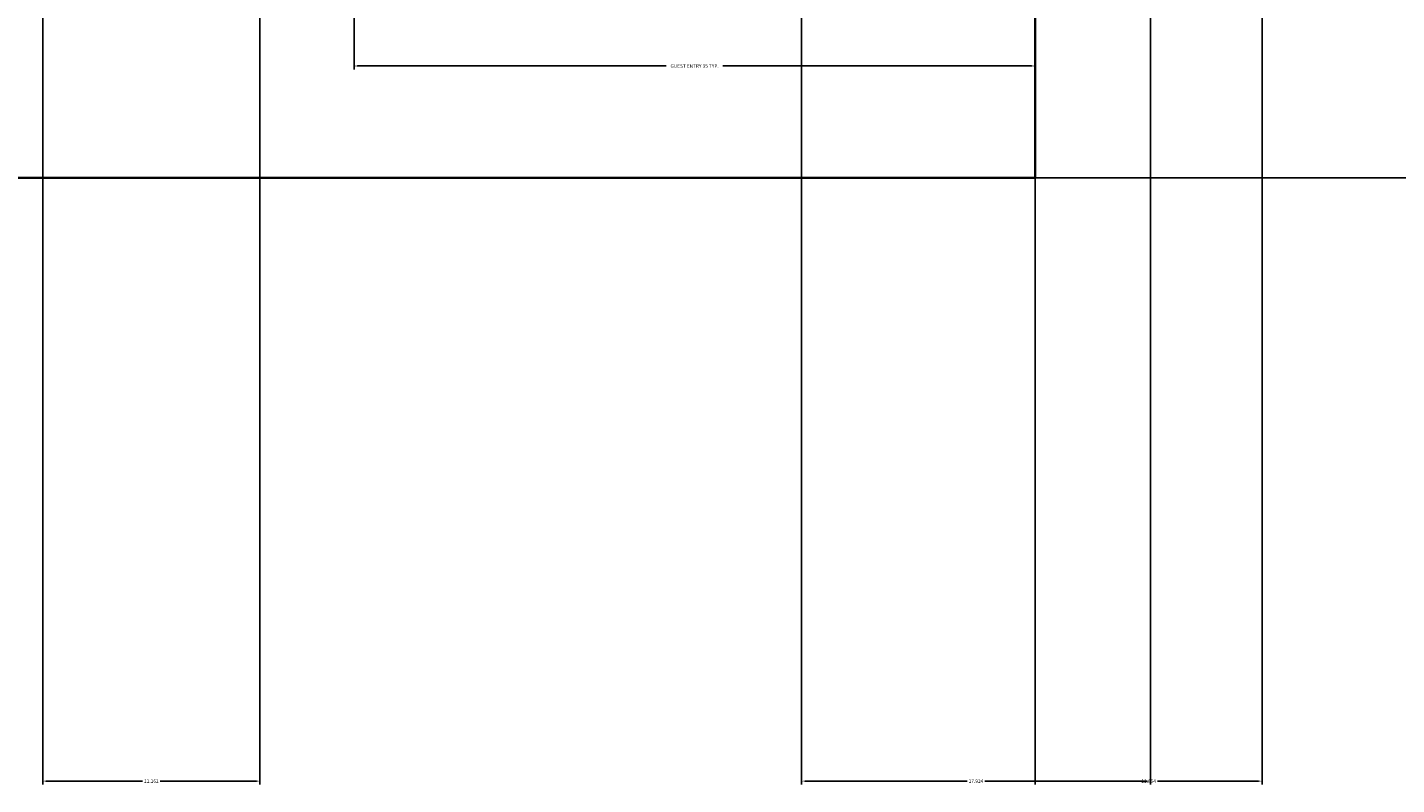
# Model space of a CAD drawing. Units: feet. Extents: x 1654 to 2985, y 1348 to 2230.
# Tile 8 of 53: x 1956 to 2027, y 1534 to 1573. Entities that reach past the tile are written whole.
import ezdxf

# ---------------------------------------------------------------- set-up
doc = ezdxf.new("R2010")
doc.units = ezdxf.units.FT
for name, color, linetype, lineweight in [('A-ANNO-DIMS', 2, 'Continuous', 18), ('A-FLOR', 7, 'Continuous', 25), ('A-WALL', 7, 'Continuous', 35)]:
    doc.layers.add(name, color=color, linetype=linetype, lineweight=lineweight)
doc.styles.get("Standard").update_dxf_attribs({"font": 'arial.ttf'})
doc.dimstyles.get("Standard").update_dxf_attribs({"dimtxt": 0.18, "dimasz": 0.18, "dimexe": 0.18, "dimexo": 0.0625, "dimgap": 0.09, "dimtad": 0, "dimtih": 1, "dimtoh": 1, "dimdec": 4, "dimzin": 0, "dimdsep": 46, "dimtxsty": 'Standard', "dimcen": 0.09, "dimadec": 0, "dimazin": 0, "dimtfac": 1, "dimtdec": 4, "dimtofl": 0, "dimtmove": 0, "dimatfit": 3, "dimfxl": 1, "dimtolj": 1, "dimtzin": 0, "dimarcsym": 0})

# ---------------------------------------------------------------- blocks, each defined once
blk = doc.blocks.new('*D30')
at = {"layer": 'A-ANNO-DIMS', "color": 0, "lineweight": -2, "transparency": 16777216}
for p, q in [((1973.092, 1576.192), (1973.092, 1570.825)), ((2008.092, 1576.192), (2008.092, 1570.825)), ((1973.272, 1571.005), (1989.137, 1571.005)), ((2007.912, 1571.005), (1992.048, 1571.005))]:
    blk.add_line(p, q, dxfattribs=at)
at = {"layer": 'A-ANNO-DIMS', "color": 0, "transparency": 16777216}
for points in [[(1973.272, 1571.035), (1973.272, 1570.975), (1973.092, 1571.005)], [(2007.912, 1571.035), (2007.912, 1570.975), (2008.092, 1571.005)]]:
    blk.add_solid(points, dxfattribs=at)
at = {"layer": 'Defpoints', "color": 0, "transparency": 16777216}
for p in [(1973.092, 1576.255), (2008.092, 1576.255), (2008.092, 1571.005)]:
    blk.add_point(p, dxfattribs=at)
at = {"layer": 'A-ANNO-DIMS', "color": 0, "transparency": 16777216, "insert": (1990.592, 1571.005), "char_height": 0.18, "attachment_point": 5}
blk.add_mtext('\\A1;GUEST ENTRY 35 TYP.', dxfattribs=at)
blk = doc.blocks.new('*D97')
at = {"layer": 'A-ANNO-DIMS', "color": 0, "lineweight": -2, "transparency": 16777216}
for p, q in [((1957.092, 2108.192), (1957.092, 1534.075)), ((1968.254, 2108.192), (1968.254, 1534.075)), ((1957.272, 1534.255), (1962.219, 1534.255)), ((1968.074, 1534.255), (1963.128, 1534.255))]:
    blk.add_line(p, q, dxfattribs=at)
at = {"layer": 'A-ANNO-DIMS', "color": 0, "transparency": 16777216}
for points in [[(1957.272, 1534.285), (1957.272, 1534.225), (1957.092, 1534.255)], [(1968.074, 1534.285), (1968.074, 1534.225), (1968.254, 1534.255)]]:
    blk.add_solid(points, dxfattribs=at)
at = {"layer": 'Defpoints', "color": 0, "transparency": 16777216}
for p in [(1957.092, 2108.255), (1968.254, 2108.255), (1968.254, 1534.255)]:
    blk.add_point(p, dxfattribs=at)
at = {"layer": 'A-ANNO-DIMS', "color": 0, "transparency": 16777216, "insert": (1962.673, 1534.255), "char_height": 0.18, "attachment_point": 5}
blk.add_mtext('\\A1;11.162', dxfattribs=at)
blk = doc.blocks.new('*D101')
at = {"layer": 'A-ANNO-DIMS', "color": 0, "lineweight": -2, "transparency": 16777216}
for p, q in [((1996.092, 2039.192), (1996.092, 1534.075)), ((2014.016, 2039.192), (2014.016, 1534.075)), ((1996.272, 1534.255), (2004.599, 1534.255)), ((2013.836, 1534.255), (2005.509, 1534.255))]:
    blk.add_line(p, q, dxfattribs=at)
at = {"layer": 'A-ANNO-DIMS', "color": 0, "transparency": 16777216}
for points in [[(1996.272, 1534.285), (1996.272, 1534.225), (1996.092, 1534.255)], [(2013.836, 1534.285), (2013.836, 1534.225), (2014.016, 1534.255)]]:
    blk.add_solid(points, dxfattribs=at)
at = {"layer": 'Defpoints', "color": 0, "transparency": 16777216}
for p in [(1996.092, 2039.255), (2014.016, 2039.255), (2014.016, 1534.255)]:
    blk.add_point(p, dxfattribs=at)
at = {"layer": 'A-ANNO-DIMS', "color": 0, "transparency": 16777216, "insert": (2005.054, 1534.255), "char_height": 0.18, "attachment_point": 5}
blk.add_mtext('\\A1;17.924', dxfattribs=at)
blk = doc.blocks.new('*D102')
at = {"layer": 'A-ANNO-DIMS', "color": 0, "lineweight": -2, "transparency": 16777216}
for p, q in [((2008.092, 1742.192), (2008.092, 1534.075)), ((2019.757, 1742.192), (2019.757, 1534.075)), ((2008.272, 1534.255), (2013.47, 1534.255)), ((2019.577, 1534.255), (2014.379, 1534.255))]:
    blk.add_line(p, q, dxfattribs=at)
at = {"layer": 'A-ANNO-DIMS', "color": 0, "transparency": 16777216}
for points in [[(2008.272, 1534.285), (2008.272, 1534.225), (2008.092, 1534.255)], [(2019.577, 1534.285), (2019.577, 1534.225), (2019.757, 1534.255)]]:
    blk.add_solid(points, dxfattribs=at)
at = {"layer": 'Defpoints', "color": 0, "transparency": 16777216}
for p in [(2008.092, 1742.255), (2019.757, 1742.255), (2019.757, 1534.255)]:
    blk.add_point(p, dxfattribs=at)
at = {"layer": 'A-ANNO-DIMS', "color": 0, "transparency": 16777216, "insert": (2013.925, 1534.255), "char_height": 0.18, "attachment_point": 5}
blk.add_mtext('\\A1;11.664', dxfattribs=at)

msp = doc.modelspace()

# ---------------------------------------------------------------- linework, layer by layer
at = {"layer": 'A-FLOR'}
msp.add_line((2008.0924, 1565.2549), (2211.0924, 1565.2549), dxfattribs=at)
at = {"layer": 'A-WALL'}
for p, q in [((2008.0924, 1565.2549), (2008.0924, 1576.2549)), ((1843.0924, 1565.2549), (2008.0924, 1565.2549))]:
    msp.add_line(p, q, dxfattribs=at)

# ---------------------------------------------------------------- dimensions: what is measured, and where the dimension line sits
at = {"layer": 'A-ANNO-DIMS'}
for base, p1, p2, picture, middle in [((1968.2542, 1534.2549), (1957.0924, 2108.2549), (1968.2542, 2108.2549), '*D97', (1962.6733, 1534.2549)), ((2014.016, 1534.2549), (1996.0924, 2039.2549), (2014.016, 2039.2549), '*D101', (2005.0542, 1534.2549)), ((2019.7567, 1534.2549), (2008.0924, 1742.2549), (2019.7567, 1742.2549), '*D102', (2013.9246, 1534.2549))]:
    dim = msp.add_linear_dim(base=base, p1=p1, p2=p2, dimstyle='Standard', override={"dimdec": 3, "dimlfac": 1, "dimrnd": 0, "dimzin": 0, "dimdsep": 46, "dimlunit": 2}, dxfattribs=at)
    dim.commit()
    dim.dimension.update_dxf_attribs({"geometry": picture, "text_midpoint": middle})
dim = msp.add_linear_dim(base=(2008.0924, 1571.0049), p1=(1973.0924, 1576.2549), p2=(2008.0924, 1576.2549), text='GUEST ENTRY <> TYP.', dimstyle='Standard', override={"dimdec": 0, "dimlfac": 1, "dimrnd": 0, "dimzin": 0, "dimdsep": 46, "dimlunit": 2}, dxfattribs=at)
dim.commit()
dim.dimension.update_dxf_attribs({"geometry": '*D30', "text_midpoint": (1990.5924, 1571.0049)})

doc.saveas('drawing.dxf')
